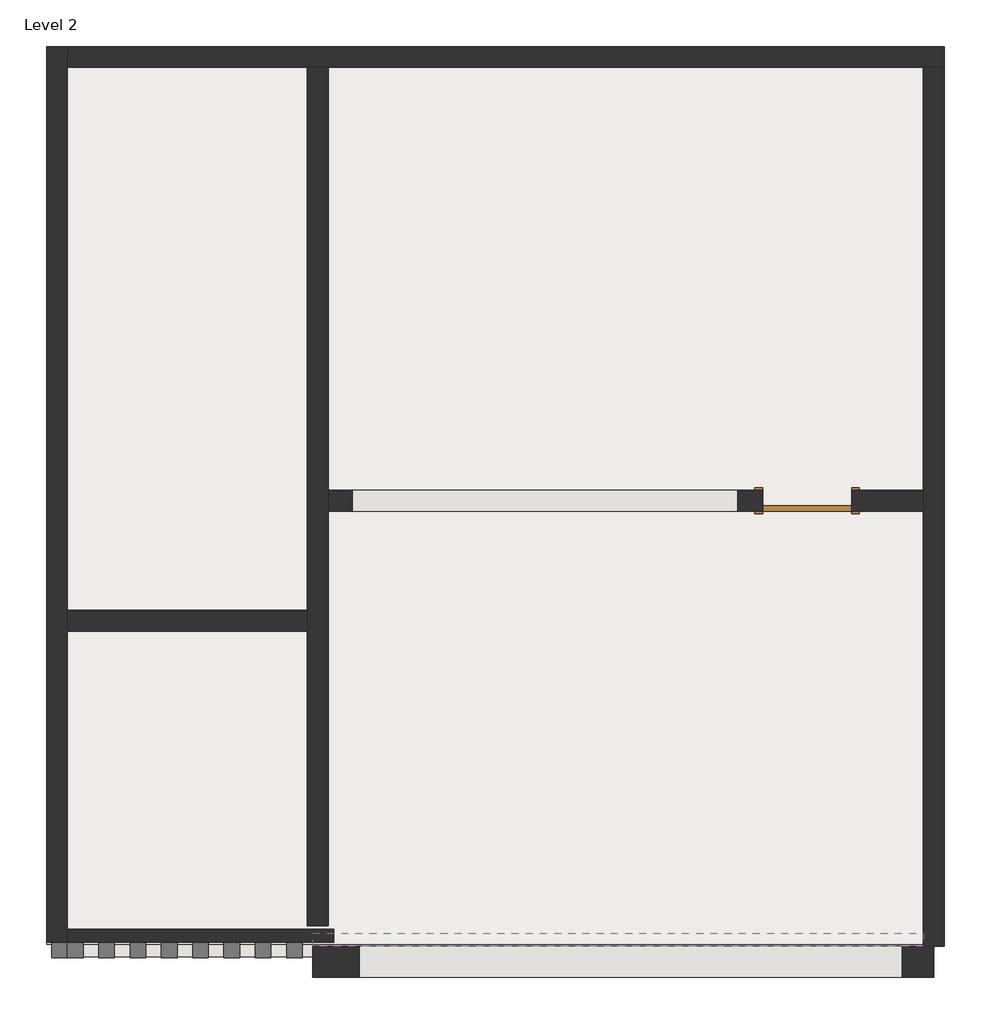
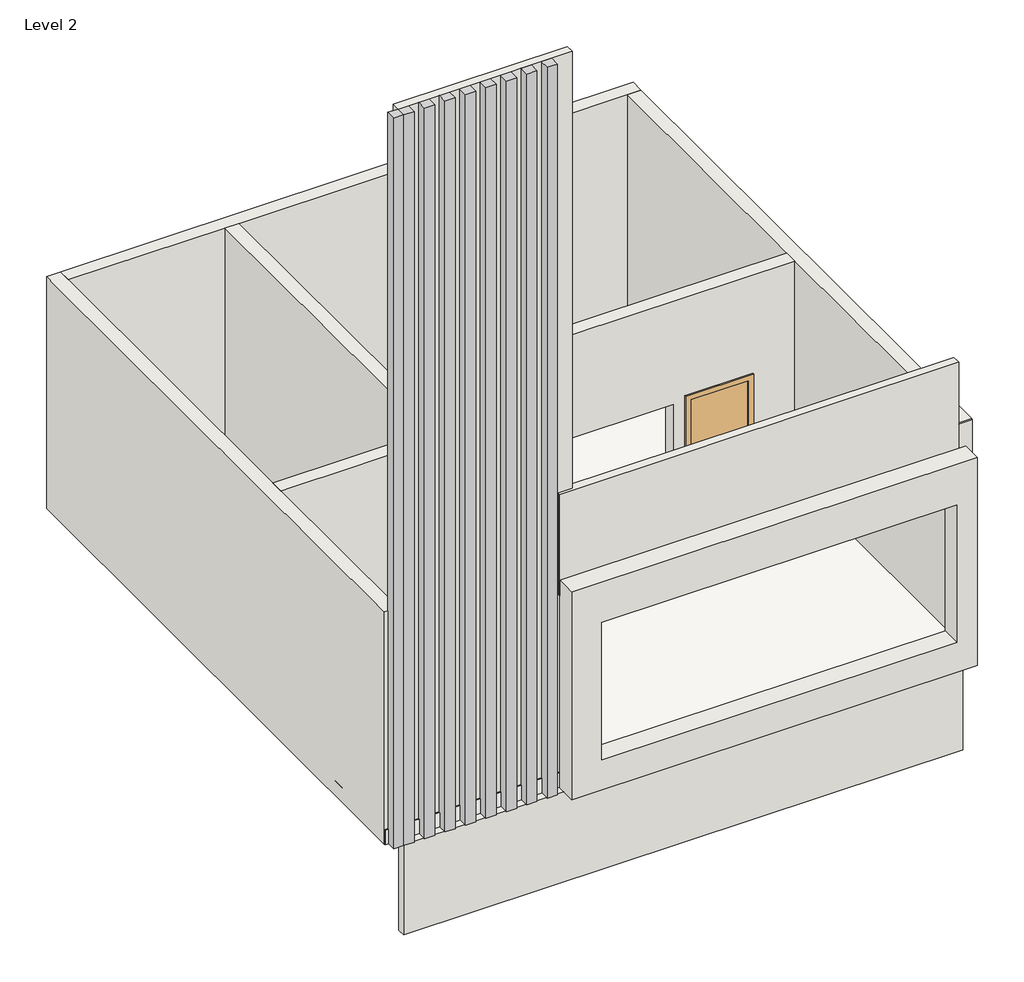
# One storey: 10 walls, 9 proxies, 1 door, 1 roof.
"""IFC4 building model written with IfcOpenShell, lengths in millimetres."""

from ifc_helpers import new_model, si_unit, frame, origin, place, context, project, spatial, polyline, outline, extrude, faceted_brep, transform, mapped, element, save
from components import door_10fd3a06, walls_1_walls_1_1a52f32e

model = new_model("IFC4")

# Units and contexts
model_context = context("Model", 3, world=origin())
ifc_project = project(units=[si_unit("LENGTHUNIT", "METRE", prefix="MILLI")], contexts=[model_context])

# Site, building, storey
site = spatial("IfcSite", under=ifc_project)
building = spatial("IfcBuilding", under=site)
storey = spatial("IfcBuildingStorey", under=building, Name="Level 2", Elevation=4572.0)

# Proxies
placement = place(None, origin())
element("IfcBuildingElementProxy", 1, Name="Cornice", ObjectType="Cornice", at=placement, inside=storey, context=model_context, shape_type="SweptSolid", body=[
    extrude(outline(polyline([(-6344.7561565, 1484.2485991), (-6344.7561565, 1331.8485991), (-6497.1561565, 1331.8485991), (-6497.1561565, 1484.2485991), (-6344.7561565, 1484.2485991)])), frame((0.0, 0.0, 4572.0), z_axis=(0.0, 0.0, 1.0), x_axis=(1.0, 0.0, 0.0)), (0.0, 0.0, 1.0), 11513.8737884),
])
element("IfcBuildingElementProxy", 2, Name="Cornice", ObjectType="Cornice", at=placement, inside=storey, context=model_context, shape_type="SweptSolid", body=[
    extrude(outline(polyline([(-6649.5561565, 1484.2485991), (-6649.5561565, 1331.8485991), (-6801.9561565, 1331.8485991), (-6801.9561565, 1484.2485991), (-6649.5561565, 1484.2485991)])), frame((0.0, 0.0, 4572.0), z_axis=(0.0, 0.0, 1.0), x_axis=(1.0, 0.0, 0.0)), (0.0, 0.0, 1.0), 11513.8737884),
])
element("IfcBuildingElementProxy", 3, Name="Cornice", ObjectType="Cornice", at=placement, inside=storey, context=model_context, shape_type="SweptSolid", body=[
    extrude(outline(polyline([(-6954.3561565, 1484.2485991), (-6954.3561565, 1331.8485991), (-7106.7561565, 1331.8485991), (-7106.7561565, 1484.2485991), (-6954.3561565, 1484.2485991)])), frame((0.0, 0.0, 4572.0), z_axis=(0.0, 0.0, 1.0), x_axis=(1.0, 0.0, 0.0)), (0.0, 0.0, 1.0), 11513.8737884),
])
element("IfcBuildingElementProxy", 4, Name="Cornice", ObjectType="Cornice", at=placement, inside=storey, context=model_context, shape_type="SweptSolid", body=[
    extrude(outline(polyline([(-7259.1561565, 1484.2485991), (-7259.1561565, 1331.8485991), (-7411.5561565, 1331.8485991), (-7411.5561565, 1484.2485991), (-7259.1561565, 1484.2485991)])), frame((0.0, 0.0, 4572.0), z_axis=(0.0, 0.0, 1.0), x_axis=(1.0, 0.0, 0.0)), (0.0, 0.0, 1.0), 11513.8737884),
])
element("IfcBuildingElementProxy", 5, Name="Cornice", ObjectType="Cornice", at=placement, inside=storey, context=model_context, shape_type="SweptSolid", body=[
    extrude(outline(polyline([(-7563.9561565, 1484.2485991), (-7563.9561565, 1331.8485991), (-7716.3561565, 1331.8485991), (-7716.3561565, 1484.2485991), (-7563.9561565, 1484.2485991)])), frame((0.0, 0.0, 4572.0), z_axis=(0.0, 0.0, 1.0), x_axis=(1.0, 0.0, 0.0)), (0.0, 0.0, 1.0), 11513.8737884),
])
element("IfcBuildingElementProxy", 6, Name="Cornice", ObjectType="Cornice", at=placement, inside=storey, context=model_context, shape_type="SweptSolid", body=[
    extrude(outline(polyline([(-7868.7561565, 1484.2485991), (-7868.7561565, 1331.8485991), (-8021.1561565, 1331.8485991), (-8021.1561565, 1484.2485991), (-7868.7561565, 1484.2485991)])), frame((0.0, 0.0, 4572.0), z_axis=(0.0, 0.0, 1.0), x_axis=(1.0, 0.0, 0.0)), (0.0, 0.0, 1.0), 11513.8737884),
])
element("IfcBuildingElementProxy", 7, Name="Cornice", ObjectType="Cornice", at=placement, inside=storey, context=model_context, shape_type="SweptSolid", body=[
    extrude(outline(polyline([(-8173.5561565, 1484.2485991), (-8173.5561565, 1331.8485991), (-8325.9561565, 1331.8485991), (-8325.9561565, 1484.2485991), (-8173.5561565, 1484.2485991)])), frame((0.0, 0.0, 4572.0), z_axis=(0.0, 0.0, 1.0), x_axis=(1.0, 0.0, 0.0)), (0.0, 0.0, 1.0), 11513.8737884),
])
element("IfcBuildingElementProxy", 8, Name="Cornice", ObjectType="Cornice", at=placement, inside=storey, context=model_context, shape_type="SweptSolid", body=[
    extrude(outline(polyline([(-8478.3561565, 1484.2485991), (-8478.3561565, 1331.8485991), (-8630.7561565, 1331.8485991), (-8630.7561565, 1484.2485991), (-8478.3561565, 1484.2485991)])), frame((0.0, 0.0, 4572.0), z_axis=(0.0, 0.0, 1.0), x_axis=(1.0, 0.0, 0.0)), (0.0, 0.0, 1.0), 11513.8737884),
])
element("IfcBuildingElementProxy", 9, Name="Cornice", ObjectType="Cornice", at=placement, inside=storey, context=model_context, shape_type="SweptSolid", body=[
    extrude(outline(polyline([(-8630.7561565, 1484.2485991), (-8630.7561565, 1331.8485991), (-8783.1561565, 1331.8485991), (-8783.1561565, 1484.2485991), (-8630.7561565, 1484.2485991)])), frame((0.0, 0.0, 4572.0), z_axis=(0.0, 0.0, 1.0), x_axis=(1.0, 0.0, 0.0)), (0.0, 0.0, 1.0), 11513.8737884),
])

# Door
door_shape = door_10fd3a06(model_context)
element("IfcDoor", 10, ObjectType="Door-Single-Panel : 34\" x 80\"", at=placement, inside=storey, context=model_context, shape_type="MappedRepresentation", body=[
    mapped(door_shape, transform((-1429.8561565, 5783.1985991, 4572.0), x_axis=(-1.0, 0.0, 0.0), y_axis=(0.0, -1.0, 0.0), z_axis=(0.0, 0.0, 1.0))),
])

# Roof
element("IfcRoof", 11, ObjectType="Generic - 9\"", at=placement, inside=storey, context=model_context, shape_type="SweptSolid", body=[
    extrude(outline(polyline([(-8833.9561565, 10202.7985991), (-96.3561565, 10202.7985991), (-96.3561565, 1465.1985991), (-8833.9561565, 1465.1985991), (-8833.9561565, 10202.7985991)])), frame((0.0, 0.0, 4572.0), z_axis=(0.0, 0.0, 1.0), x_axis=(1.0, 0.0, 0.0)), (0.0, 0.0, 1.0), 228.6),
])

# Walls
element("IfcWall", 12, ObjectType="Generic - 5\"", at=placement, inside=storey, context=model_context, shape_type="Brep", body=[
    faceted_brep([(-6039.9561565, 1611.2485991, 4572.0), (-8630.7561565, 1611.2485991, 4572.0), (-8630.7561565, 1611.2485991, 16085.8737884), (-6039.9561565, 1611.2485991, 16085.8737884), (-6039.9561565, 1484.2485991, 4572.0), (-6039.9561565, 1484.2485991, 16085.8737884), (-8630.7561565, 1484.2485991, 16085.8737884), (-8630.7561565, 1484.2485991, 15544.8), (-8630.7561565, 1484.2485991, 11887.2), (-8630.7561565, 1484.2485991, 8229.6), (-8630.7561565, 1484.2485991, 4572.0)], [[[0, 1, 2, 3]], [[4, 5, 6, 7, 8, 9, 10]], [[1, 0, 4, 10]], [[3, 2, 6, 5]], [[0, 3, 5, 4]], [[1, 10, 9, 8, 7, 6, 2]]]),
])
element("IfcWall", 13, ObjectType="Generic - 5\"", at=placement, inside=storey, context=model_context, shape_type="Brep", body=[
    faceted_brep([(-8630.7561565, 1344.5485991, 3154.9356368), (-299.5561565, 1344.5485991, 3154.9356368), (-299.5561565, 1344.5485991, 4572.0), (-8630.7561565, 1344.5485991, 4572.0), (-8630.7561565, 1471.5485991, 3154.9356368), (-8630.7561565, 1471.5485991, 4572.0), (-299.5561565, 1471.5485991, 4572.0), (-299.5561565, 1471.5485991, 3154.9356368), (-8630.7561565, 1465.1985991, 4572.0)], [[[0, 1, 2, 3]], [[4, 5, 6, 7]], [[1, 0, 4, 7]], [[3, 2, 6, 5, 8]], [[1, 7, 6, 2]], [[0, 3, 8, 5, 4]]]),
])
element("IfcWall", 14, ObjectType="Generic - 5\"", at=placement, inside=storey, context=model_context, shape_type="Brep", body=[
    faceted_brep([(-299.5561565, 1573.1485991, 9201.3855951), (-299.5561565, 1573.1485991, 7601.9769391), (-6243.1561565, 1573.1485991, 7601.9769391), (-6243.1561565, 1573.1485991, 9201.3855951), (-299.5561565, 1446.1485991, 7601.9769391), (-299.5561565, 1446.1485991, 8229.6), (-299.5561565, 1446.1485991, 9201.3855951), (-6243.1561565, 1446.1485991, 9201.3855951), (-6243.1561565, 1446.1485991, 7601.9769391)], [[[0, 1, 2, 3]], [[4, 5, 6, 7, 8]], [[2, 1, 4, 8]], [[3, 2, 8, 7]], [[0, 3, 7, 6]], [[0, 6, 5, 4, 1]]]),
])
element("IfcWall", 15, ObjectType="Generic - 8\"", at=placement, inside=storey, context=model_context, shape_type="SweptSolid", body=[
    extrude(outline(polyline([(-6293.9561565, 4513.1985991), (-8630.7561565, 4513.1985991), (-8630.7561565, 4716.3985991), (-6293.9561565, 4716.3985991), (-6293.9561565, 4513.1985991)])), frame((0.0, 0.0, 4572.0), z_axis=(0.0, 0.0, 1.0), x_axis=(1.0, 0.0, 0.0)), (0.0, 0.0, 1.0), 3657.6),
])
element("IfcWall", 16, ObjectType="Generic - 8\"", at=placement, inside=storey, context=model_context, shape_type="Brep", body=[
    faceted_brep([(-6293.9561565, 9999.5985991, 4572.0), (-6293.9561565, 4716.3985991, 4572.0), (-6293.9561565, 4513.1985991, 4572.0), (-6293.9561565, 1642.9985991, 4572.0), (-6293.9561565, 1642.9985991, 8229.6), (-6293.9561565, 4513.1985991, 8229.6), (-6293.9561565, 4716.3985991, 8229.6), (-6293.9561565, 9999.5985991, 8229.6), (-6090.7561565, 9999.5985991, 4572.0), (-6090.7561565, 9999.5985991, 8229.6), (-6090.7561565, 5884.7985991, 8229.6), (-6090.7561565, 5681.5985991, 8229.6), (-6090.7561565, 1642.9985991, 8229.6), (-6090.7561565, 1642.9985991, 4572.0), (-6090.7561565, 5681.5985991, 4572.0), (-6090.7561565, 5884.7985991, 4572.0)], [[[0, 1, 2, 3, 4, 5, 6, 7]], [[8, 9, 10, 11, 12, 13, 14, 15]], [[3, 2, 1, 0, 8, 15, 14, 13]], [[4, 3, 13, 12]], [[7, 6, 5, 4, 12, 11, 10, 9]], [[0, 7, 9, 8]]]),
])
element("IfcWall", 17, ObjectType="Generic - 8\"", at=placement, inside=storey, context=model_context, shape_type="SweptSolid", body=[
    extrude(outline(polyline([(4572.0, -6090.7561565), (4572.0, -1861.6561565), (6604.0, -1861.6561565), (6604.0, -998.0561565), (4572.0, -998.0561565), (4572.0, -299.5561565), (8229.6, -299.5561565), (8229.6, -6090.7561565), (4572.0, -6090.7561565)]), holes=[polyline([(6598.408423, -2105.8901764), (4837.1392215, -2105.8901764), (4837.1392215, -5855.9012139), (6598.408423, -5855.9012139), (6598.408423, -2105.8901764)])]), frame((0.0, 5681.5985991, 0.0), z_axis=(0.0, 1.0, 0.0), x_axis=(0.0, 0.0, 1.0)), (0.0, 0.0, 1.0), 203.2),
])
element("IfcWall", 18, ObjectType="Generic - 8\"", at=placement, inside=storey, context=model_context, shape_type="Brep", body=[
    faceted_brep([(-299.5561565, 9999.5985991, 4572.0), (-299.5561565, 5884.7985991, 4572.0), (-299.5561565, 5681.5985991, 4572.0), (-299.5561565, 1446.1485991, 4572.0), (-299.5561565, 1446.1485991, 7601.9769391), (-299.5561565, 1446.1485991, 8229.6), (-299.5561565, 1465.1985991, 8229.6), (-299.5561565, 5681.5985991, 8229.6), (-299.5561565, 5884.7985991, 8229.6), (-299.5561565, 9999.5985991, 8229.6), (-96.3561565, 9999.5985991, 4572.0), (-96.3561565, 9999.5985991, 8229.6), (-96.3561565, 1465.1985991, 8229.6), (-96.3561565, 1446.1485991, 8229.6), (-96.3561565, 1446.1485991, 4572.0)], [[[0, 1, 2, 3, 4, 5, 6, 7, 8, 9]], [[10, 11, 12, 13, 14]], [[3, 2, 1, 0, 10, 14]], [[6, 5, 13, 12]], [[9, 8, 7, 6, 12, 11]], [[5, 4, 3, 14, 13]], [[0, 9, 11, 10]]]),
])
element("IfcWall", 19, ObjectType="Generic - 8\"", at=placement, inside=storey, context=model_context, shape_type="Brep", body=[
    faceted_brep([(-8630.7561565, 1484.2485991, 4572.0), (-8630.7561565, 1611.2485991, 4572.0), (-8630.7561565, 4513.1985991, 4572.0), (-8630.7561565, 4716.3985991, 4572.0), (-8630.7561565, 9999.5985991, 4572.0), (-8630.7561565, 10202.7985991, 4572.0), (-8630.7561565, 10202.7985991, 8229.6), (-8630.7561565, 9999.5985991, 8229.6), (-8630.7561565, 4716.3985991, 8229.6), (-8630.7561565, 4513.1985991, 8229.6), (-8630.7561565, 1484.2485991, 8229.6), (-8833.9561565, 1484.2485991, 4572.0), (-8833.9561565, 1484.2485991, 8229.6), (-8833.9561565, 9999.5985991, 8229.6), (-8833.9561565, 10202.7985991, 8229.6), (-8833.9561565, 10202.7985991, 4572.0)], [[[0, 1, 2, 3, 4, 5, 6, 7, 8, 9, 10]], [[11, 12, 13, 14, 15]], [[5, 4, 3, 2, 1, 0, 11, 15]], [[10, 9, 8, 7, 6, 14, 13, 12]], [[0, 10, 12, 11]], [[6, 5, 15, 14]]]),
])
element("IfcWall", 20, ObjectType="Generic - 8\"", at=placement, inside=storey, context=model_context, shape_type="Brep", body=[
    faceted_brep([(-8630.7561565, 9999.5985991, 4572.0), (-6293.9561565, 9999.5985991, 4572.0), (-6090.7561565, 9999.5985991, 4572.0), (-299.5561565, 9999.5985991, 4572.0), (-96.3561565, 9999.5985991, 4572.0), (-96.3561565, 9999.5985991, 8229.6), (-299.5561565, 9999.5985991, 8229.6), (-6090.7561565, 9999.5985991, 8229.6), (-6293.9561565, 9999.5985991, 8229.6), (-8630.7561565, 9999.5985991, 8229.6), (-8630.7561565, 10202.7985991, 4572.0), (-8630.7561565, 10202.7985991, 8229.6), (-96.3561565, 10202.7985991, 8229.6), (-96.3561565, 10202.7985991, 4572.0)], [[[0, 1, 2, 3, 4, 5, 6, 7, 8, 9]], [[10, 11, 12, 13]], [[4, 3, 2, 1, 0, 10, 13]], [[9, 8, 7, 6, 5, 12, 11]], [[0, 9, 11, 10]], [[5, 4, 13, 12]]]),
])
walls_1_walls_1_shape = walls_1_walls_1_1a52f32e(model_context)
element("IfcWall", 21, ObjectType="Walls 1 : Walls 1", at=placement, inside=storey, context=model_context, shape_type="MappedRepresentation", body=[
    mapped(walls_1_walls_1_shape, transform((0.0, 0.0, 0.0), x_axis=(1.0, 0.0, 0.0), y_axis=(0.0, 1.0, 0.0), z_axis=(0.0, 0.0, 1.0))),
])

save(model, "model.ifc")

# Revit data of these elements
# Type "Door-Single-Panel : 34\" x 80\""
#   Type Mark = "8"
#   Construction Type Id = "DOOR"
#   Assembly Code = "C1020300"
#   Analytic Construction = "Wooden"
#   Thickness = 0' - 2"
#   Thermal Resistance (R) = 2.5876 (h·ft²·°F)/BTU
#   Swing Angle [instance default] = 90.00°
#   Heat Transfer Coefficient (U) = 0.3865 BTU/(h·ft²·°F)
#   Height = 6' - 8"
#   Trim Projection Ext = 0' - 1"
#   Trim Projection Int = 0' - 1"
#   Trim Width = 0' - 3"
#   Width = 2' - 10"
#   Define Thermal Properties by = 1
#   Panel Material = Wood - Birch - Solid Stained Light Low Gloss
#   Trim Material = Paint - Sienna
#   Visual Light Transmittance = 0
#   Solar Heat Gain Coefficient = 0
#   Function = (empty or 0)
#   Wall Closure = (empty or 0)
# Type "Generic - 9\""
#   Assembly Code = "B1020"
#   Layers, outside or top first: 0' - 9" no material (function 1)
# Type "Generic - 5\""
#   Assembly Code = "B2010"
#   Layers, outside or top first: 0' - 5" no material (function 1)
# Type "Generic - 8\""
#   Assembly Code = "B2010"
#   Layers, outside or top first: 0' - 8" no material (function 1)
# Elements 1, 2, 3, 4, 5, 6, 7, 8, 9 (IfcBuildingElementProxy, "Cornice")
#   Phase Created = New Construction
#   Materials on its faces: "Default Wall"
# Element 10 (IfcDoor, "Door-Single-Panel : 34\" x 80\"")
#   Swing Angle = 90.00°
#   Phase Created = New Construction
#   Materials on its faces: "Paint - Sienna", "Wood - Birch - Solid Stained Light Low Gloss"
# Element 11 (IfcRoof, "Generic - 9\"")
#   built-in parameter 1001705 = 15.75 (stored number, unit not read)
#   built-in parameter 1001710 = 33615
#   Phase Created = New Construction
#   Materials on its faces: "Default Roof"
# Element 12 (IfcWall, "Generic - 5\"")
#   Top Offset = 25' - 9.30212"
#   Base Offset = 0' - 0"
#   wall height = 37' - 9.30212"
#   Phase Created = New Construction
#   Base Constraint = Level 2
#   Top Constraint = Level 3
#   Materials on its faces: "Default Wall"
# Element 13 (IfcWall, "Generic - 5\"")
#   built-in parameter 1001111 = -4' - 7.78994"
#   Top Offset = -12' - 0"
#   Base Offset = -4' - 7.78994"
#   wall height = 4' - 7.78994"
#   Phase Created = New Construction
#   Base Constraint = Level 2
#   Top Constraint = Level 3
#   Materials on its faces: "Default Wall"
# Element 14 (IfcWall, "Generic - 5\"")
#   built-in parameter 1001111 = 9' - 11.29043"
#   Top Offset = 3' - 2.25928"
#   Base Offset = 9' - 11.29043"
#   wall height = 5' - 2.96884"
#   Phase Created = New Construction
#   Base Constraint = Level 2
#   Top Constraint = Level 3
#   Materials on its faces: "Default Wall"
# Elements 15, 16, 17, 18, 19, 20 (IfcWall, "Generic - 8\"")
#   Top Offset = 0' - 0"
#   Base Offset = 0' - 0"
#   Unconnected Height = 12' - 0"
#   wall height = 12' - 0"
#   Phase Created = New Construction
#   Base Constraint = Level 2
#   Materials on its faces: "Default Wall"
# Element 21 (IfcWall, "Walls 1 : Walls 1")
#   Phase Created = New Construction
#   Materials on its faces: "Default Wall"
# Materials
#   "Wood - Birch - Solid Stained Light Low Gloss": class "Wood", colour RGB 210 159 95, transparency 0, Cost = 0
#   "Paint - Sienna": colour RGB 118 70 51, transparency 0, Cost = 0
#   "Default Wall": colour RGB 128 128 128, transparency 0
#   "Default Roof": colour RGB 88 101 114, transparency 0
